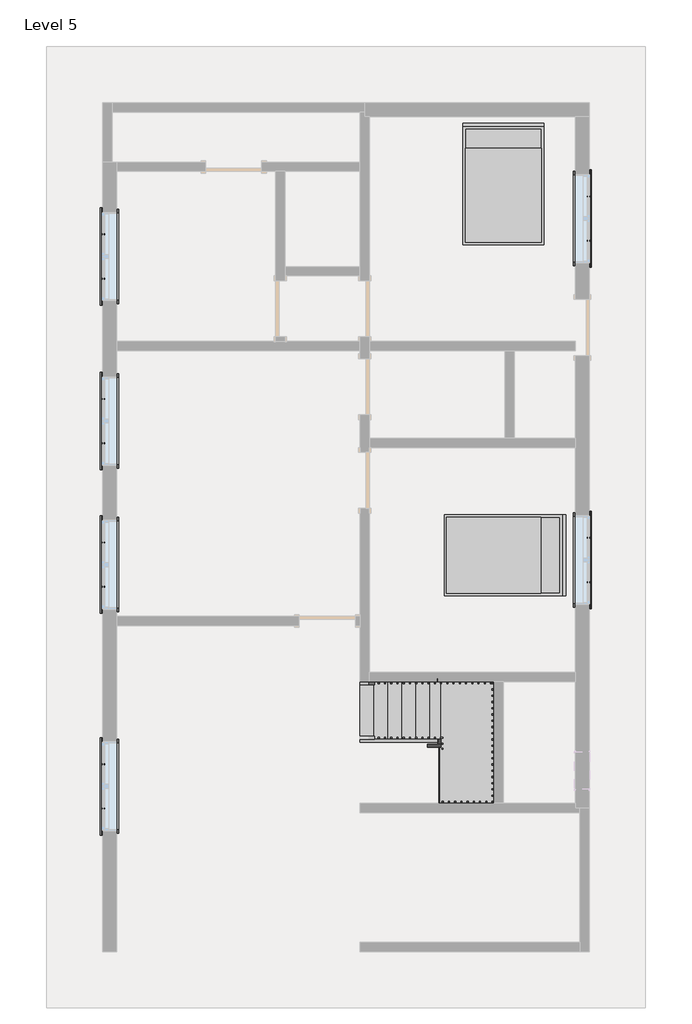
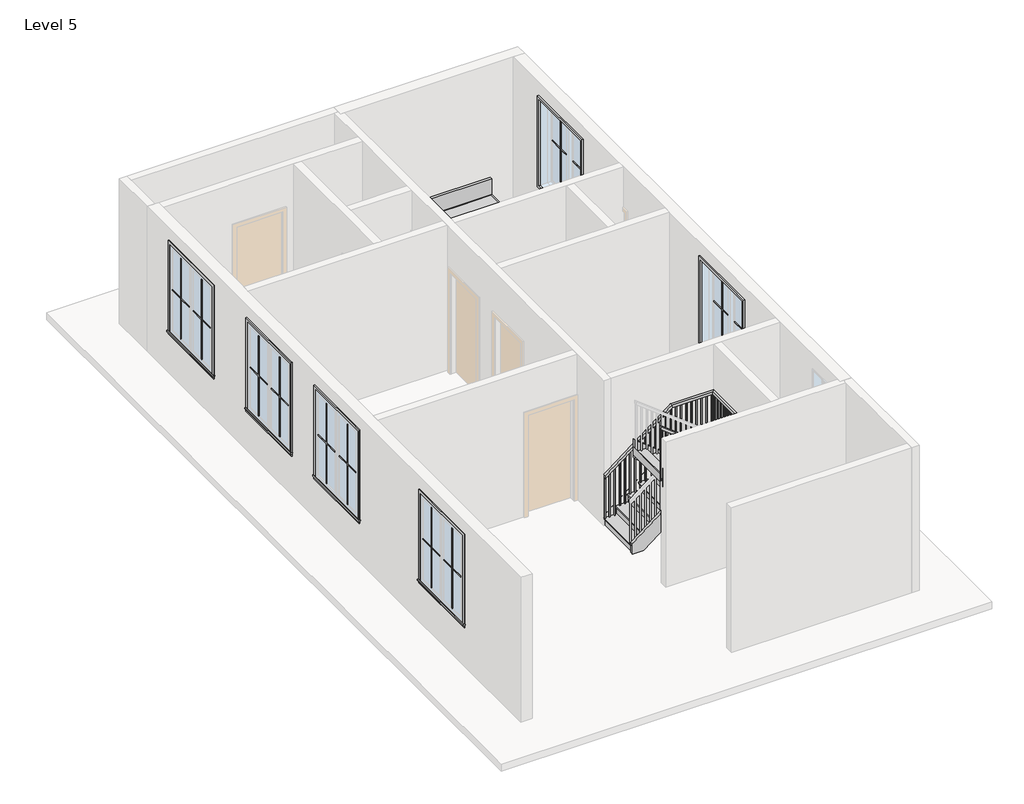
# One storey, part 2 of 2: 24 proxies, 6 members, 2 furniture elements, 1 railing, 1 stair flight.
"""IFC4 building model written with IfcOpenShell, lengths in millimetres."""

from ifc_helpers import new_model, si_unit, frame, origin, place, context, project, spatial, polyline, outline, extrude, faceted_brep, transform, mapped, element, save
from components import muntin_pattern_2x2_muntin_pattern_2x2_bff912c5, muntin_pattern_2x2_muntin_pattern_2x2_c2194282, trim_window_exterior_flat_with_sill_e04b3088, trim_window_interior_flat_picture_frame_2a7685fe, bed_17739_bed_17739_15c61121, stair_flight_8cfd25ce

model = new_model("IFC4")

# Units and contexts
model_context = context("Model", 3, world=origin())
ifc_project = project(units=[si_unit("LENGTHUNIT", "METRE", prefix="MILLI")], contexts=[model_context])

# Site, building, storey
site = spatial("IfcSite", under=ifc_project)
building = spatial("IfcBuilding", under=site)
storey = spatial("IfcBuildingStorey", under=building, Name="Level 5", Elevation=9601.2)

# Proxies
placement = place(None, origin())
muntin_pattern_2x2_muntin_pattern_2x2_shape = muntin_pattern_2x2_muntin_pattern_2x2_bff912c5(model_context)
element("IfcBuildingElementProxy", 1, Name="Muntin Pattern_2x2 : Muntin Pattern_2x2", ObjectType="Muntin Pattern_2x2 : Muntin Pattern_2x2", at=placement, inside=storey, context=model_context, shape_type="MappedRepresentation", body=[
    mapped(muntin_pattern_2x2_muntin_pattern_2x2_shape, transform((-5204.1165352, 3633.8812696, 10585.45), x_axis=(0.0, 1.0, 0.0), y_axis=(-1.0, 0.0, 0.0), z_axis=(0.0, 0.0, 1.0))),
])
element("IfcBuildingElementProxy", 2, Name="Muntin Pattern_2x2 : Muntin Pattern_2x2", ObjectType="Muntin Pattern_2x2 : Muntin Pattern_2x2", at=placement, inside=storey, context=model_context, shape_type="MappedRepresentation", body=[
    mapped(muntin_pattern_2x2_muntin_pattern_2x2_shape, transform((2701.6334648, 4971.3355313, 10585.45), x_axis=(0.0, -1.0, 0.0), y_axis=(1.0, 0.0, 0.0), z_axis=(0.0, 0.0, 1.0))),
])
element("IfcBuildingElementProxy", 3, Name="Muntin Pattern_2x2 : Muntin Pattern_2x2", ObjectType="Muntin Pattern_2x2 : Muntin Pattern_2x2", at=placement, inside=storey, context=model_context, shape_type="MappedRepresentation", body=[
    mapped(muntin_pattern_2x2_muntin_pattern_2x2_shape, transform((2701.6334648, -584.9144687, 10585.45), x_axis=(0.0, -1.0, 0.0), y_axis=(1.0, 0.0, 0.0), z_axis=(0.0, 0.0, 1.0))),
])
element("IfcBuildingElementProxy", 4, Name="Muntin Pattern_2x2 : Muntin Pattern_2x2", ObjectType="Muntin Pattern_2x2 : Muntin Pattern_2x2", at=placement, inside=storey, context=model_context, shape_type="MappedRepresentation", body=[
    mapped(muntin_pattern_2x2_muntin_pattern_2x2_shape, transform((-5204.1165352, 954.9605313, 10585.45), x_axis=(0.0, 1.0, 0.0), y_axis=(-1.0, 0.0, 0.0), z_axis=(0.0, 0.0, 1.0))),
])
element("IfcBuildingElementProxy", 5, Name="Muntin Pattern_2x2 : Muntin Pattern_2x2", ObjectType="Muntin Pattern_2x2 : Muntin Pattern_2x2", at=placement, inside=storey, context=model_context, shape_type="MappedRepresentation", body=[
    mapped(muntin_pattern_2x2_muntin_pattern_2x2_shape, transform((-5204.1165352, -1381.8394687, 10585.45), x_axis=(0.0, 1.0, 0.0), y_axis=(-1.0, 0.0, 0.0), z_axis=(0.0, 0.0, 1.0))),
])
element("IfcBuildingElementProxy", 6, Name="Muntin Pattern_2x2 : Muntin Pattern_2x2", ObjectType="Muntin Pattern_2x2 : Muntin Pattern_2x2", at=placement, inside=storey, context=model_context, shape_type="MappedRepresentation", body=[
    mapped(muntin_pattern_2x2_muntin_pattern_2x2_shape, transform((-5204.1165352, -4988.6394687, 10585.45), x_axis=(0.0, 1.0, 0.0), y_axis=(-1.0, 0.0, 0.0), z_axis=(0.0, 0.0, 1.0))),
])
muntin_pattern_2x2_muntin_pattern_2x2_2_shape = muntin_pattern_2x2_muntin_pattern_2x2_c2194282(model_context)
element("IfcBuildingElementProxy", 7, Name="Muntin Pattern_2x2 : Muntin Pattern_2x2", ObjectType="Muntin Pattern_2x2 : Muntin Pattern_2x2", at=placement, inside=storey, context=model_context, shape_type="MappedRepresentation", body=[
    mapped(muntin_pattern_2x2_muntin_pattern_2x2_2_shape, transform((-5204.1165352, 4354.6062696, 10585.45), x_axis=(0.0, -1.0, 0.0), y_axis=(1.0, 0.0, 0.0), z_axis=(0.0, 0.0, 1.0))),
])
element("IfcBuildingElementProxy", 8, Name="Muntin Pattern_2x2 : Muntin Pattern_2x2", ObjectType="Muntin Pattern_2x2 : Muntin Pattern_2x2", at=placement, inside=storey, context=model_context, shape_type="MappedRepresentation", body=[
    mapped(muntin_pattern_2x2_muntin_pattern_2x2_2_shape, transform((2701.6334648, 4250.6105313, 10585.45), x_axis=(0.0, 1.0, 0.0), y_axis=(-1.0, 0.0, 0.0), z_axis=(0.0, 0.0, 1.0))),
])
element("IfcBuildingElementProxy", 9, Name="Muntin Pattern_2x2 : Muntin Pattern_2x2", ObjectType="Muntin Pattern_2x2 : Muntin Pattern_2x2", at=placement, inside=storey, context=model_context, shape_type="MappedRepresentation", body=[
    mapped(muntin_pattern_2x2_muntin_pattern_2x2_2_shape, transform((2701.6334648, -1305.6394687, 10585.45), x_axis=(0.0, 1.0, 0.0), y_axis=(-1.0, 0.0, 0.0), z_axis=(0.0, 0.0, 1.0))),
])
element("IfcBuildingElementProxy", 10, Name="Muntin Pattern_2x2 : Muntin Pattern_2x2", ObjectType="Muntin Pattern_2x2 : Muntin Pattern_2x2", at=placement, inside=storey, context=model_context, shape_type="MappedRepresentation", body=[
    mapped(muntin_pattern_2x2_muntin_pattern_2x2_2_shape, transform((-5204.1165352, 1675.6855313, 10585.45), x_axis=(0.0, -1.0, 0.0), y_axis=(1.0, 0.0, 0.0), z_axis=(0.0, 0.0, 1.0))),
])
element("IfcBuildingElementProxy", 11, Name="Muntin Pattern_2x2 : Muntin Pattern_2x2", ObjectType="Muntin Pattern_2x2 : Muntin Pattern_2x2", at=placement, inside=storey, context=model_context, shape_type="MappedRepresentation", body=[
    mapped(muntin_pattern_2x2_muntin_pattern_2x2_2_shape, transform((-5204.1165352, -661.1144687, 10585.45), x_axis=(0.0, -1.0, 0.0), y_axis=(1.0, 0.0, 0.0), z_axis=(0.0, 0.0, 1.0))),
])
element("IfcBuildingElementProxy", 12, Name="Muntin Pattern_2x2 : Muntin Pattern_2x2", ObjectType="Muntin Pattern_2x2 : Muntin Pattern_2x2", at=placement, inside=storey, context=model_context, shape_type="MappedRepresentation", body=[
    mapped(muntin_pattern_2x2_muntin_pattern_2x2_2_shape, transform((-5204.1165352, -4267.9144687, 10585.45), x_axis=(0.0, -1.0, 0.0), y_axis=(1.0, 0.0, 0.0), z_axis=(0.0, 0.0, 1.0))),
])
trim_window_exterior_flat_with_sill_shape = trim_window_exterior_flat_with_sill_e04b3088(model_context)
element("IfcBuildingElementProxy", 13, Name="Trim-Window-Exterior-Flat : with Sill", ObjectType="Trim-Window-Exterior-Flat : with Sill", at=placement, inside=storey, context=model_context, shape_type="MappedRepresentation", body=[
    mapped(trim_window_exterior_flat_with_sill_shape, transform((-5213.6415352, 3994.2437696, 12344.4), x_axis=(0.0, -1.0, 0.0), y_axis=(0.0, 0.0, 1.0), z_axis=(-1.0, 0.0, 0.0))),
])
element("IfcBuildingElementProxy", 14, Name="Trim-Window-Exterior-Flat : with Sill", ObjectType="Trim-Window-Exterior-Flat : with Sill", at=placement, inside=storey, context=model_context, shape_type="MappedRepresentation", body=[
    mapped(trim_window_exterior_flat_with_sill_shape, transform((2711.1584648, 4610.9730313, 12344.4), x_axis=(0.0, 1.0, 0.0), y_axis=(0.0, 0.0, 1.0), z_axis=(1.0, 0.0, 0.0))),
])
element("IfcBuildingElementProxy", 15, Name="Trim-Window-Exterior-Flat : with Sill", ObjectType="Trim-Window-Exterior-Flat : with Sill", at=placement, inside=storey, context=model_context, shape_type="MappedRepresentation", body=[
    mapped(trim_window_exterior_flat_with_sill_shape, transform((2711.1584648, -945.2769687, 12344.4), x_axis=(0.0, 1.0, 0.0), y_axis=(0.0, 0.0, 1.0), z_axis=(1.0, 0.0, 0.0))),
])
element("IfcBuildingElementProxy", 16, Name="Trim-Window-Exterior-Flat : with Sill", ObjectType="Trim-Window-Exterior-Flat : with Sill", at=placement, inside=storey, context=model_context, shape_type="MappedRepresentation", body=[
    mapped(trim_window_exterior_flat_with_sill_shape, transform((-5213.6415352, 1315.3230313, 12344.4), x_axis=(0.0, -1.0, 0.0), y_axis=(0.0, 0.0, 1.0), z_axis=(-1.0, 0.0, 0.0))),
])
element("IfcBuildingElementProxy", 17, Name="Trim-Window-Exterior-Flat : with Sill", ObjectType="Trim-Window-Exterior-Flat : with Sill", at=placement, inside=storey, context=model_context, shape_type="MappedRepresentation", body=[
    mapped(trim_window_exterior_flat_with_sill_shape, transform((-5213.6415352, -1021.4769687, 12344.4), x_axis=(0.0, -1.0, 0.0), y_axis=(0.0, 0.0, 1.0), z_axis=(-1.0, 0.0, 0.0))),
])
element("IfcBuildingElementProxy", 18, Name="Trim-Window-Exterior-Flat : with Sill", ObjectType="Trim-Window-Exterior-Flat : with Sill", at=placement, inside=storey, context=model_context, shape_type="MappedRepresentation", body=[
    mapped(trim_window_exterior_flat_with_sill_shape, transform((-5213.6415352, -4628.2769687, 12344.4), x_axis=(0.0, -1.0, 0.0), y_axis=(0.0, 0.0, 1.0), z_axis=(-1.0, 0.0, 0.0))),
])
trim_window_interior_flat_picture_frame_shape = trim_window_interior_flat_picture_frame_2a7685fe(model_context)
element("IfcBuildingElementProxy", 19, Name="Trim-Window-Interior-Flat : Picture Frame", ObjectType="Trim-Window-Interior-Flat : Picture Frame", at=placement, inside=storey, context=model_context, shape_type="MappedRepresentation", body=[
    mapped(trim_window_interior_flat_picture_frame_shape, transform((-4985.0415352, 3994.2437696, 12344.4), x_axis=(0.0, 1.0, 0.0), y_axis=(0.0, 0.0, 1.0), z_axis=(1.0, 0.0, 0.0))),
])
element("IfcBuildingElementProxy", 20, Name="Trim-Window-Interior-Flat : Picture Frame", ObjectType="Trim-Window-Interior-Flat : Picture Frame", at=placement, inside=storey, context=model_context, shape_type="MappedRepresentation", body=[
    mapped(trim_window_interior_flat_picture_frame_shape, transform((2482.5584648, 4610.9730313, 12344.4), x_axis=(0.0, -1.0, 0.0), y_axis=(0.0, 0.0, 1.0), z_axis=(-1.0, 0.0, 0.0))),
])
element("IfcBuildingElementProxy", 21, Name="Trim-Window-Interior-Flat : Picture Frame", ObjectType="Trim-Window-Interior-Flat : Picture Frame", at=placement, inside=storey, context=model_context, shape_type="MappedRepresentation", body=[
    mapped(trim_window_interior_flat_picture_frame_shape, transform((2482.5584648, -945.2769687, 12344.4), x_axis=(0.0, -1.0, 0.0), y_axis=(0.0, 0.0, 1.0), z_axis=(-1.0, 0.0, 0.0))),
])
element("IfcBuildingElementProxy", 22, Name="Trim-Window-Interior-Flat : Picture Frame", ObjectType="Trim-Window-Interior-Flat : Picture Frame", at=placement, inside=storey, context=model_context, shape_type="MappedRepresentation", body=[
    mapped(trim_window_interior_flat_picture_frame_shape, transform((-4985.0415352, 1315.3230313, 12344.4), x_axis=(0.0, 1.0, 0.0), y_axis=(0.0, 0.0, 1.0), z_axis=(1.0, 0.0, 0.0))),
])
element("IfcBuildingElementProxy", 23, Name="Trim-Window-Interior-Flat : Picture Frame", ObjectType="Trim-Window-Interior-Flat : Picture Frame", at=placement, inside=storey, context=model_context, shape_type="MappedRepresentation", body=[
    mapped(trim_window_interior_flat_picture_frame_shape, transform((-4985.0415352, -1021.4769687, 12344.4), x_axis=(0.0, 1.0, 0.0), y_axis=(0.0, 0.0, 1.0), z_axis=(1.0, 0.0, 0.0))),
])
element("IfcBuildingElementProxy", 24, Name="Trim-Window-Interior-Flat : Picture Frame", ObjectType="Trim-Window-Interior-Flat : Picture Frame", at=placement, inside=storey, context=model_context, shape_type="MappedRepresentation", body=[
    mapped(trim_window_interior_flat_picture_frame_shape, transform((-4985.0415352, -4628.2769687, 12344.4), x_axis=(0.0, 1.0, 0.0), y_axis=(0.0, 0.0, 1.0), z_axis=(1.0, 0.0, 0.0))),
])

# Furniture
bed_17739_bed_17739_shape = bed_17739_bed_17739_15c61121(model_context)
element("IfcFurniture", 25, ObjectType="Bed_17739 : Bed_17739", at=placement, inside=storey, context=model_context, shape_type="MappedRepresentation", body=[
    mapped(bed_17739_bed_17739_shape, transform((1314.1584648, 5149.1645078, 9601.2), x_axis=(1.0, 0.0, 0.0), y_axis=(0.0, 1.0, 0.0), z_axis=(0.0, 0.0, 1.0))),
])
element("IfcFurniture", 26, ObjectType="Bed_17739 : Bed_17739", at=placement, inside=storey, context=model_context, shape_type="MappedRepresentation", body=[
    mapped(bed_17739_bed_17739_shape, transform((1314.1584648, -869.0769687, 9601.2), x_axis=(0.0, -1.0, 0.0), y_axis=(1.0, 0.0, 0.0), z_axis=(0.0, 0.0, 1.0))),
])

# Members
element("IfcMember", 27, ObjectType="Stringer - 2\" Width", at=placement, inside=storey, context=model_context, shape_type="SweptSolid", body=[
    extrude(outline(polyline([(9822.9399812, -1022.6415352), (9601.2, -1022.6415352), (9601.2, -811.2687863), (10862.7333333, 810.8400359), (10862.7333333, 314.3488758), (9822.9399812, -1022.6415352)])), frame((0.0, -2926.4769687, 0.0), z_axis=(0.0, 1.0, 0.0), x_axis=(0.0, 0.0, 1.0)), (0.0, 0.0, 1.0), 50.8),
])
element("IfcMember", 28, ObjectType="Stringer - 2\" Width", at=placement, inside=storey, context=model_context, shape_type="SweptSolid", body=[
    extrude(outline(polyline([(1161.7584648, -2875.6769687), (1212.5584648, -2875.6769687), (1212.5584648, -4907.6769687), (1161.7584648, -4907.6769687), (1161.7584648, -2875.6769687)])), frame((0.0, 0.0, 10557.9333333), z_axis=(0.0, 0.0, 1.0), x_axis=(1.0, 0.0, 0.0)), (0.0, 0.0, 1.0), 304.8),
])
element("IfcMember", 29, ObjectType="Stringer - 2\" Width", at=placement, inside=storey, context=model_context, shape_type="SweptSolid", body=[
    extrude(outline(polyline([(10557.9333333, 884.5469698), (12041.1765283, -1022.6415352), (11655.0494451, -1022.6415352), (10557.9333333, 388.0558097), (10557.9333333, 884.5469698)])), frame((0.0, -4958.4769687, 0.0), z_axis=(0.0, 1.0, 0.0), x_axis=(0.0, 0.0, 1.0)), (0.0, 0.0, 1.0), 50.8),
])
element("IfcMember", 30, ObjectType="Stringer - 2\" Width", at=placement, inside=storey, context=model_context, shape_type="SweptSolid", body=[
    extrude(outline(polyline([(9822.9399812, -1022.6415352), (9601.2, -1022.6415352), (9601.2, -811.2687863), (10421.7567404, 243.8221038), (10807.8838236, 243.8221038), (9822.9399812, -1022.6415352)])), frame((0.0, -3912.0539367, 0.0), z_axis=(0.0, 1.0, 0.0), x_axis=(0.0, 0.0, 1.0)), (0.0, 0.0, 1.0), 50.8),
])
element("IfcMember", 31, ObjectType="Stringer - 2\" Width", at=placement, inside=storey, context=model_context, shape_type="SweptSolid", body=[
    extrude(outline(polyline([(243.8221038, -3861.2539367), (294.6221038, -3861.2539367), (294.6221038, -3942.4769687), (243.8221038, -3942.4769687), (243.8221038, -3861.2539367)])), frame((0.0, 0.0, 10557.9333333), z_axis=(0.0, 0.0, 1.0), x_axis=(1.0, 0.0, 0.0)), (0.0, 0.0, 1.0), 304.8),
])
element("IfcMember", 32, ObjectType="Stringer - 2\" Width", at=placement, inside=storey, context=model_context, shape_type="SweptSolid", body=[
    extrude(outline(polyline([(10630.5978382, 294.6221038), (11016.7249214, 294.6221038), (12041.1765283, -1022.6415352), (11655.0494451, -1022.6415352), (10630.5978382, 294.6221038)])), frame((0.0, -3993.2769687, 0.0), z_axis=(0.0, 1.0, 0.0), x_axis=(0.0, 0.0, 1.0)), (0.0, 0.0, 1.0), 50.8),
])

# Railing
element("IfcRailing", 33, ObjectType="Handrail - Rectangular", at=placement, inside=storey, context=model_context, shape_type="SolidModel", body=[
    faceted_brep([(-1022.6415352, -2926.4769687, 10684.9333333), (-1022.6415352, -2926.4769687, 10620.7783974), (-1022.6415352, -2977.2769687, 10620.7783974), (-1022.6415352, -2977.2769687, 10684.9333333), (294.6221038, -2926.4769687, 11700.9333333), (311.9370364, -2926.4769687, 11650.1333333), (311.9370364, -2977.2769687, 11650.1333333), (294.6221038, -2977.2769687, 11700.9333333), (1161.7584648, -2926.4769687, 11700.9333333), (1161.7584648, -2926.4769687, 11650.1333333), (1110.9584648, -2977.2769687, 11650.1333333), (1110.9584648, -2977.2769687, 11700.9333333), (1161.7584648, -4907.6769687, 11700.9333333), (1161.7584648, -4907.6769687, 11650.1333333), (1110.9584648, -4856.8769687, 11650.1333333), (1110.9584648, -4856.8769687, 11700.9333333), (514.1660437, -4907.6769687, 11700.9333333), (496.8511111, -4907.6769687, 11650.1333333), (496.8511111, -4856.8769687, 11650.1333333), (514.1660437, -4856.8769687, 11700.9333333), (-1022.6415352, -4907.6769687, 12886.2666667), (-1022.6415352, -4856.8769687, 12886.2666667), (-1022.6415352, -4856.8769687, 12822.1117307), (-1022.6415352, -4907.6769687, 12822.1117307)], [[[0, 1, 2, 3]], [[1, 0, 4, 5]], [[2, 1, 5, 6]], [[3, 2, 6, 7]], [[0, 3, 7, 4]], [[5, 4, 8, 9]], [[6, 5, 9, 10]], [[7, 6, 10, 11]], [[4, 7, 11, 8]], [[9, 8, 12, 13]], [[10, 9, 13, 14]], [[11, 10, 14, 15]], [[8, 11, 15, 12]], [[13, 12, 16, 17]], [[14, 13, 17, 18]], [[15, 14, 18, 19]], [[12, 15, 19, 16]], [[20, 21, 22, 23]], [[17, 16, 20, 23]], [[18, 17, 23, 22]], [[19, 18, 22, 21]], [[16, 19, 21, 20]]]),
    extrude(outline(polyline([(12809.8674089, -1006.7665352), (11802.5333333, -1006.7665352), (11802.5333333, -987.7165352), (12795.1742226, -987.7165352), (12809.8674089, -1006.7665352)])), frame((0.0, -4891.8019687, 0.0), z_axis=(0.0, 1.0, 0.0), x_axis=(0.0, 0.0, 1.0)), (0.0, 0.0, 1.0), 19.05),
    extrude(outline(polyline([(12731.5037488, -905.1665352), (11802.5333333, -905.1665352), (11802.5333333, -886.1165352), (12716.8105626, -886.1165352), (12731.5037488, -905.1665352)])), frame((0.0, -4891.8019687, 0.0), z_axis=(0.0, 1.0, 0.0), x_axis=(0.0, 0.0, 1.0)), (0.0, 0.0, 1.0), 19.05),
    extrude(outline(polyline([(12653.1400888, -803.5665352), (11802.5333333, -803.5665352), (11802.5333333, -784.5165352), (12638.4469025, -784.5165352), (12653.1400888, -803.5665352)])), frame((0.0, -4891.8019687, 0.0), z_axis=(0.0, 1.0, 0.0), x_axis=(0.0, 0.0, 1.0)), (0.0, 0.0, 1.0), 19.05),
    extrude(outline(polyline([(12574.7764287, -701.9665352), (11633.2, -701.9665352), (11633.2, -682.9165352), (12560.0832425, -682.9165352), (12574.7764287, -701.9665352)])), frame((0.0, -4891.8019687, 0.0), z_axis=(0.0, 1.0, 0.0), x_axis=(0.0, 0.0, 1.0)), (0.0, 0.0, 1.0), 19.05),
    extrude(outline(polyline([(12496.4127687, -600.3665352), (11633.2, -600.3665352), (11633.2, -581.3165352), (12481.7195824, -581.3165352), (12496.4127687, -600.3665352)])), frame((0.0, -4891.8019687, 0.0), z_axis=(0.0, 1.0, 0.0), x_axis=(0.0, 0.0, 1.0)), (0.0, 0.0, 1.0), 19.05),
    extrude(outline(polyline([(12418.0491086, -498.7665352), (11463.8666667, -498.7665352), (11463.8666667, -479.7165352), (12403.3559224, -479.7165352), (12418.0491086, -498.7665352)])), frame((0.0, -4891.8019687, 0.0), z_axis=(0.0, 1.0, 0.0), x_axis=(0.0, 0.0, 1.0)), (0.0, 0.0, 1.0), 19.05),
    extrude(outline(polyline([(12339.6854486, -397.1665352), (11463.8666667, -397.1665352), (11463.8666667, -378.1165352), (12324.9922623, -378.1165352), (12339.6854486, -397.1665352)])), frame((0.0, -4891.8019687, 0.0), z_axis=(0.0, 1.0, 0.0), x_axis=(0.0, 0.0, 1.0)), (0.0, 0.0, 1.0), 19.05),
    extrude(outline(polyline([(12261.3217885, -295.5665352), (11294.5333333, -295.5665352), (11294.5333333, -276.5165352), (12246.6286023, -276.5165352), (12261.3217885, -295.5665352)])), frame((0.0, -4891.8019687, 0.0), z_axis=(0.0, 1.0, 0.0), x_axis=(0.0, 0.0, 1.0)), (0.0, 0.0, 1.0), 19.05),
    extrude(outline(polyline([(12182.9581285, -193.9665352), (11294.5333333, -193.9665352), (11294.5333333, -174.9165352), (12168.2649422, -174.9165352), (12182.9581285, -193.9665352)])), frame((0.0, -4891.8019687, 0.0), z_axis=(0.0, 1.0, 0.0), x_axis=(0.0, 0.0, 1.0)), (0.0, 0.0, 1.0), 19.05),
    extrude(outline(polyline([(12104.5944684, -92.3665352), (11125.2, -92.3665352), (11125.2, -73.3165352), (12089.9012822, -73.3165352), (12104.5944684, -92.3665352)])), frame((0.0, -4891.8019687, 0.0), z_axis=(0.0, 1.0, 0.0), x_axis=(0.0, 0.0, 1.0)), (0.0, 0.0, 1.0), 19.05),
    extrude(outline(polyline([(12026.2308084, 9.2334648), (11125.2, 9.2334648), (11125.2, 28.2834648), (12011.5376221, 28.2834648), (12026.2308084, 9.2334648)])), frame((0.0, -4891.8019687, 0.0), z_axis=(0.0, 1.0, 0.0), x_axis=(0.0, 0.0, 1.0)), (0.0, 0.0, 1.0), 19.05),
    extrude(outline(polyline([(11947.8671484, 110.8334648), (11125.2, 110.8334648), (11125.2, 129.8834648), (11933.1739621, 129.8834648), (11947.8671484, 110.8334648)])), frame((0.0, -4891.8019687, 0.0), z_axis=(0.0, 1.0, 0.0), x_axis=(0.0, 0.0, 1.0)), (0.0, 0.0, 1.0), 19.05),
    extrude(outline(polyline([(11869.5034883, 212.4334648), (10955.8666667, 212.4334648), (10955.8666667, 231.4834648), (11854.8103021, 231.4834648), (11869.5034883, 212.4334648)])), frame((0.0, -4891.8019687, 0.0), z_axis=(0.0, 1.0, 0.0), x_axis=(0.0, 0.0, 1.0)), (0.0, 0.0, 1.0), 19.05),
    extrude(outline(polyline([(11791.1398283, 314.0334648), (10786.5333333, 314.0334648), (10786.5333333, 333.0834648), (11776.446642, 333.0834648), (11791.1398283, 314.0334648)])), frame((0.0, -4891.8019687, 0.0), z_axis=(0.0, 1.0, 0.0), x_axis=(0.0, 0.0, 1.0)), (0.0, 0.0, 1.0), 19.05),
    extrude(outline(polyline([(11712.7761682, 415.6334648), (10786.5333333, 415.6334648), (10786.5333333, 434.6834648), (11698.082982, 434.6834648), (11712.7761682, 415.6334648)])), frame((0.0, -4891.8019687, 0.0), z_axis=(0.0, 1.0, 0.0), x_axis=(0.0, 0.0, 1.0)), (0.0, 0.0, 1.0), 19.05),
    extrude(outline(polyline([(536.2834648, -4891.8019687), (517.2334648, -4891.8019687), (517.2334648, -4872.7519687), (536.2834648, -4872.7519687), (536.2834648, -4891.8019687)])), frame((0.0, 0.0, 10786.5333333), z_axis=(0.0, 0.0, 1.0), x_axis=(1.0, 0.0, 0.0)), (0.0, 0.0, 1.0), 863.6),
    extrude(outline(polyline([(637.8834648, -4891.8019687), (618.8334648, -4891.8019687), (618.8334648, -4872.7519687), (637.8834648, -4872.7519687), (637.8834648, -4891.8019687)])), frame((0.0, 0.0, 10786.5333333), z_axis=(0.0, 0.0, 1.0), x_axis=(1.0, 0.0, 0.0)), (0.0, 0.0, 1.0), 863.6),
    extrude(outline(polyline([(739.4834648, -4891.8019687), (720.4334648, -4891.8019687), (720.4334648, -4872.7519687), (739.4834648, -4872.7519687), (739.4834648, -4891.8019687)])), frame((0.0, 0.0, 10786.5333333), z_axis=(0.0, 0.0, 1.0), x_axis=(1.0, 0.0, 0.0)), (0.0, 0.0, 1.0), 863.6),
    extrude(outline(polyline([(841.0834648, -4891.8019687), (822.0334648, -4891.8019687), (822.0334648, -4872.7519687), (841.0834648, -4872.7519687), (841.0834648, -4891.8019687)])), frame((0.0, 0.0, 10786.5333333), z_axis=(0.0, 0.0, 1.0), x_axis=(1.0, 0.0, 0.0)), (0.0, 0.0, 1.0), 863.6),
    extrude(outline(polyline([(942.6834648, -4891.8019687), (923.6334648, -4891.8019687), (923.6334648, -4872.7519687), (942.6834648, -4872.7519687), (942.6834648, -4891.8019687)])), frame((0.0, 0.0, 10786.5333333), z_axis=(0.0, 0.0, 1.0), x_axis=(1.0, 0.0, 0.0)), (0.0, 0.0, 1.0), 863.6),
    extrude(outline(polyline([(1044.2834648, -4891.8019687), (1025.2334648, -4891.8019687), (1025.2334648, -4872.7519687), (1044.2834648, -4872.7519687), (1044.2834648, -4891.8019687)])), frame((0.0, 0.0, 10786.5333333), z_axis=(0.0, 0.0, 1.0), x_axis=(1.0, 0.0, 0.0)), (0.0, 0.0, 1.0), 863.6),
    extrude(outline(polyline([(1145.8834648, -4771.1519687), (1145.8834648, -4790.2019687), (1126.8334648, -4790.2019687), (1126.8334648, -4771.1519687), (1145.8834648, -4771.1519687)])), frame((0.0, 0.0, 10786.5333333), z_axis=(0.0, 0.0, 1.0), x_axis=(1.0, 0.0, 0.0)), (0.0, 0.0, 1.0), 863.6),
    extrude(outline(polyline([(1145.8834648, -4669.5519687), (1145.8834648, -4688.6019687), (1126.8334648, -4688.6019687), (1126.8334648, -4669.5519687), (1145.8834648, -4669.5519687)])), frame((0.0, 0.0, 10786.5333333), z_axis=(0.0, 0.0, 1.0), x_axis=(1.0, 0.0, 0.0)), (0.0, 0.0, 1.0), 863.6),
    extrude(outline(polyline([(1145.8834648, -4567.9519687), (1145.8834648, -4587.0019687), (1126.8334648, -4587.0019687), (1126.8334648, -4567.9519687), (1145.8834648, -4567.9519687)])), frame((0.0, 0.0, 10786.5333333), z_axis=(0.0, 0.0, 1.0), x_axis=(1.0, 0.0, 0.0)), (0.0, 0.0, 1.0), 863.6),
    extrude(outline(polyline([(1145.8834648, -4466.3519687), (1145.8834648, -4485.4019687), (1126.8334648, -4485.4019687), (1126.8334648, -4466.3519687), (1145.8834648, -4466.3519687)])), frame((0.0, 0.0, 10786.5333333), z_axis=(0.0, 0.0, 1.0), x_axis=(1.0, 0.0, 0.0)), (0.0, 0.0, 1.0), 863.6),
    extrude(outline(polyline([(1145.8834648, -4364.7519687), (1145.8834648, -4383.8019687), (1126.8334648, -4383.8019687), (1126.8334648, -4364.7519687), (1145.8834648, -4364.7519687)])), frame((0.0, 0.0, 10786.5333333), z_axis=(0.0, 0.0, 1.0), x_axis=(1.0, 0.0, 0.0)), (0.0, 0.0, 1.0), 863.6),
    extrude(outline(polyline([(1145.8834648, -4263.1519687), (1145.8834648, -4282.2019687), (1126.8334648, -4282.2019687), (1126.8334648, -4263.1519687), (1145.8834648, -4263.1519687)])), frame((0.0, 0.0, 10786.5333333), z_axis=(0.0, 0.0, 1.0), x_axis=(1.0, 0.0, 0.0)), (0.0, 0.0, 1.0), 863.6),
    extrude(outline(polyline([(1145.8834648, -4161.5519687), (1145.8834648, -4180.6019687), (1126.8334648, -4180.6019687), (1126.8334648, -4161.5519687), (1145.8834648, -4161.5519687)])), frame((0.0, 0.0, 10786.5333333), z_axis=(0.0, 0.0, 1.0), x_axis=(1.0, 0.0, 0.0)), (0.0, 0.0, 1.0), 863.6),
    extrude(outline(polyline([(1145.8834648, -4059.9519687), (1145.8834648, -4079.0019687), (1126.8334648, -4079.0019687), (1126.8334648, -4059.9519687), (1145.8834648, -4059.9519687)])), frame((0.0, 0.0, 10786.5333333), z_axis=(0.0, 0.0, 1.0), x_axis=(1.0, 0.0, 0.0)), (0.0, 0.0, 1.0), 863.6),
    extrude(outline(polyline([(1145.8834648, -3958.3519687), (1145.8834648, -3977.4019687), (1126.8334648, -3977.4019687), (1126.8334648, -3958.3519687), (1145.8834648, -3958.3519687)])), frame((0.0, 0.0, 10786.5333333), z_axis=(0.0, 0.0, 1.0), x_axis=(1.0, 0.0, 0.0)), (0.0, 0.0, 1.0), 863.6),
    extrude(outline(polyline([(1145.8834648, -3856.7519687), (1145.8834648, -3875.8019687), (1126.8334648, -3875.8019687), (1126.8334648, -3856.7519687), (1145.8834648, -3856.7519687)])), frame((0.0, 0.0, 10786.5333333), z_axis=(0.0, 0.0, 1.0), x_axis=(1.0, 0.0, 0.0)), (0.0, 0.0, 1.0), 863.6),
    extrude(outline(polyline([(1145.8834648, -3755.1519687), (1145.8834648, -3774.2019687), (1126.8334648, -3774.2019687), (1126.8334648, -3755.1519687), (1145.8834648, -3755.1519687)])), frame((0.0, 0.0, 10786.5333333), z_axis=(0.0, 0.0, 1.0), x_axis=(1.0, 0.0, 0.0)), (0.0, 0.0, 1.0), 863.6),
    extrude(outline(polyline([(1145.8834648, -3653.5519687), (1145.8834648, -3672.6019687), (1126.8334648, -3672.6019687), (1126.8334648, -3653.5519687), (1145.8834648, -3653.5519687)])), frame((0.0, 0.0, 10786.5333333), z_axis=(0.0, 0.0, 1.0), x_axis=(1.0, 0.0, 0.0)), (0.0, 0.0, 1.0), 863.6),
    extrude(outline(polyline([(1145.8834648, -3551.9519687), (1145.8834648, -3571.0019687), (1126.8334648, -3571.0019687), (1126.8334648, -3551.9519687), (1145.8834648, -3551.9519687)])), frame((0.0, 0.0, 10786.5333333), z_axis=(0.0, 0.0, 1.0), x_axis=(1.0, 0.0, 0.0)), (0.0, 0.0, 1.0), 863.6),
    extrude(outline(polyline([(1145.8834648, -3450.3519687), (1145.8834648, -3469.4019687), (1126.8334648, -3469.4019687), (1126.8334648, -3450.3519687), (1145.8834648, -3450.3519687)])), frame((0.0, 0.0, 10786.5333333), z_axis=(0.0, 0.0, 1.0), x_axis=(1.0, 0.0, 0.0)), (0.0, 0.0, 1.0), 863.6),
    extrude(outline(polyline([(1145.8834648, -3348.7519687), (1145.8834648, -3367.8019687), (1126.8334648, -3367.8019687), (1126.8334648, -3348.7519687), (1145.8834648, -3348.7519687)])), frame((0.0, 0.0, 10786.5333333), z_axis=(0.0, 0.0, 1.0), x_axis=(1.0, 0.0, 0.0)), (0.0, 0.0, 1.0), 863.6),
    extrude(outline(polyline([(1145.8834648, -3247.1519687), (1145.8834648, -3266.2019687), (1126.8334648, -3266.2019687), (1126.8334648, -3247.1519687), (1145.8834648, -3247.1519687)])), frame((0.0, 0.0, 10786.5333333), z_axis=(0.0, 0.0, 1.0), x_axis=(1.0, 0.0, 0.0)), (0.0, 0.0, 1.0), 863.6),
    extrude(outline(polyline([(1145.8834648, -3145.5519687), (1145.8834648, -3164.6019687), (1126.8334648, -3164.6019687), (1126.8334648, -3145.5519687), (1145.8834648, -3145.5519687)])), frame((0.0, 0.0, 10786.5333333), z_axis=(0.0, 0.0, 1.0), x_axis=(1.0, 0.0, 0.0)), (0.0, 0.0, 1.0), 863.6),
    extrude(outline(polyline([(1145.8834648, -3043.9519687), (1145.8834648, -3063.0019687), (1126.8334648, -3063.0019687), (1126.8334648, -3043.9519687), (1145.8834648, -3043.9519687)])), frame((0.0, 0.0, 10786.5333333), z_axis=(0.0, 0.0, 1.0), x_axis=(1.0, 0.0, 0.0)), (0.0, 0.0, 1.0), 863.6),
    extrude(outline(polyline([(1101.4334648, -2942.3519687), (1120.4834648, -2942.3519687), (1120.4834648, -2961.4019687), (1101.4334648, -2961.4019687), (1101.4334648, -2942.3519687)])), frame((0.0, 0.0, 10786.5333333), z_axis=(0.0, 0.0, 1.0), x_axis=(1.0, 0.0, 0.0)), (0.0, 0.0, 1.0), 863.6),
    extrude(outline(polyline([(999.8334648, -2942.3519687), (1018.8834648, -2942.3519687), (1018.8834648, -2961.4019687), (999.8334648, -2961.4019687), (999.8334648, -2942.3519687)])), frame((0.0, 0.0, 10786.5333333), z_axis=(0.0, 0.0, 1.0), x_axis=(1.0, 0.0, 0.0)), (0.0, 0.0, 1.0), 863.6),
    extrude(outline(polyline([(898.2334648, -2942.3519687), (917.2834648, -2942.3519687), (917.2834648, -2961.4019687), (898.2334648, -2961.4019687), (898.2334648, -2942.3519687)])), frame((0.0, 0.0, 10786.5333333), z_axis=(0.0, 0.0, 1.0), x_axis=(1.0, 0.0, 0.0)), (0.0, 0.0, 1.0), 863.6),
    extrude(outline(polyline([(796.6334648, -2942.3519687), (815.6834648, -2942.3519687), (815.6834648, -2961.4019687), (796.6334648, -2961.4019687), (796.6334648, -2942.3519687)])), frame((0.0, 0.0, 10786.5333333), z_axis=(0.0, 0.0, 1.0), x_axis=(1.0, 0.0, 0.0)), (0.0, 0.0, 1.0), 863.6),
    extrude(outline(polyline([(695.0334648, -2942.3519687), (714.0834648, -2942.3519687), (714.0834648, -2961.4019687), (695.0334648, -2961.4019687), (695.0334648, -2942.3519687)])), frame((0.0, 0.0, 10786.5333333), z_axis=(0.0, 0.0, 1.0), x_axis=(1.0, 0.0, 0.0)), (0.0, 0.0, 1.0), 863.6),
    extrude(outline(polyline([(593.4334648, -2942.3519687), (612.4834648, -2942.3519687), (612.4834648, -2961.4019687), (593.4334648, -2961.4019687), (593.4334648, -2942.3519687)])), frame((0.0, 0.0, 10786.5333333), z_axis=(0.0, 0.0, 1.0), x_axis=(1.0, 0.0, 0.0)), (0.0, 0.0, 1.0), 863.6),
    extrude(outline(polyline([(491.8334648, -2942.3519687), (510.8834648, -2942.3519687), (510.8834648, -2961.4019687), (491.8334648, -2961.4019687), (491.8334648, -2942.3519687)])), frame((0.0, 0.0, 10786.5333333), z_axis=(0.0, 0.0, 1.0), x_axis=(1.0, 0.0, 0.0)), (0.0, 0.0, 1.0), 863.6),
    extrude(outline(polyline([(390.2334648, -2942.3519687), (409.2834648, -2942.3519687), (409.2834648, -2961.4019687), (390.2334648, -2961.4019687), (390.2334648, -2942.3519687)])), frame((0.0, 0.0, 10786.5333333), z_axis=(0.0, 0.0, 1.0), x_axis=(1.0, 0.0, 0.0)), (0.0, 0.0, 1.0), 863.6),
    extrude(outline(polyline([(288.6334648, -2942.3519687), (307.6834648, -2942.3519687), (307.6834648, -2961.4019687), (288.6334648, -2961.4019687), (288.6334648, -2942.3519687)])), frame((0.0, 0.0, 10786.5333333), z_axis=(0.0, 0.0, 1.0), x_axis=(1.0, 0.0, 0.0)), (0.0, 0.0, 1.0), 863.6),
    extrude(outline(polyline([(11553.7957248, 187.0334648), (10617.2, 187.0334648), (10617.2, 206.0834648), (11568.4889111, 206.0834648), (11553.7957248, 187.0334648)])), frame((0.0, -2961.4019687, 0.0), z_axis=(0.0, 1.0, 0.0), x_axis=(0.0, 0.0, 1.0)), (0.0, 0.0, 1.0), 19.05),
    extrude(outline(polyline([(11475.4320648, 85.4334648), (10447.8666667, 85.4334648), (10447.8666667, 104.4834648), (11490.125251, 104.4834648), (11475.4320648, 85.4334648)])), frame((0.0, -2961.4019687, 0.0), z_axis=(0.0, 1.0, 0.0), x_axis=(0.0, 0.0, 1.0)), (0.0, 0.0, 1.0), 19.05),
    extrude(outline(polyline([(11397.0684047, -16.1665352), (10447.8666667, -16.1665352), (10447.8666667, 2.8834648), (11411.761591, 2.8834648), (11397.0684047, -16.1665352)])), frame((0.0, -2961.4019687, 0.0), z_axis=(0.0, 1.0, 0.0), x_axis=(0.0, 0.0, 1.0)), (0.0, 0.0, 1.0), 19.05),
    extrude(outline(polyline([(11318.7047447, -117.7665352), (10447.8666667, -117.7665352), (10447.8666667, -98.7165352), (11333.3979309, -98.7165352), (11318.7047447, -117.7665352)])), frame((0.0, -2961.4019687, 0.0), z_axis=(0.0, 1.0, 0.0), x_axis=(0.0, 0.0, 1.0)), (0.0, 0.0, 1.0), 19.05),
    extrude(outline(polyline([(11240.3410846, -219.3665352), (10278.5333333, -219.3665352), (10278.5333333, -200.3165352), (11255.0342709, -200.3165352), (11240.3410846, -219.3665352)])), frame((0.0, -2961.4019687, 0.0), z_axis=(0.0, 1.0, 0.0), x_axis=(0.0, 0.0, 1.0)), (0.0, 0.0, 1.0), 19.05),
    extrude(outline(polyline([(11161.9774246, -320.9665352), (10278.5333333, -320.9665352), (10278.5333333, -301.9165352), (11176.6706109, -301.9165352), (11161.9774246, -320.9665352)])), frame((0.0, -2961.4019687, 0.0), z_axis=(0.0, 1.0, 0.0), x_axis=(0.0, 0.0, 1.0)), (0.0, 0.0, 1.0), 19.05),
    extrude(outline(polyline([(11083.6137645, -422.5665352), (10109.2, -422.5665352), (10109.2, -403.5165352), (11098.3069508, -403.5165352), (11083.6137645, -422.5665352)])), frame((0.0, -2961.4019687, 0.0), z_axis=(0.0, 1.0, 0.0), x_axis=(0.0, 0.0, 1.0)), (0.0, 0.0, 1.0), 19.05),
    extrude(outline(polyline([(11005.2501045, -524.1665352), (10109.2, -524.1665352), (10109.2, -505.1165352), (11019.9432908, -505.1165352), (11005.2501045, -524.1665352)])), frame((0.0, -2961.4019687, 0.0), z_axis=(0.0, 1.0, 0.0), x_axis=(0.0, 0.0, 1.0)), (0.0, 0.0, 1.0), 19.05),
    extrude(outline(polyline([(10926.8864445, -625.7665352), (9939.8666667, -625.7665352), (9939.8666667, -606.7165352), (10941.5796307, -606.7165352), (10926.8864445, -625.7665352)])), frame((0.0, -2961.4019687, 0.0), z_axis=(0.0, 1.0, 0.0), x_axis=(0.0, 0.0, 1.0)), (0.0, 0.0, 1.0), 19.05),
    extrude(outline(polyline([(10848.5227844, -727.3665352), (9939.8666667, -727.3665352), (9939.8666667, -708.3165352), (10863.2159707, -708.3165352), (10848.5227844, -727.3665352)])), frame((0.0, -2961.4019687, 0.0), z_axis=(0.0, 1.0, 0.0), x_axis=(0.0, 0.0, 1.0)), (0.0, 0.0, 1.0), 19.05),
    extrude(outline(polyline([(10770.1591244, -828.9665352), (9770.5333333, -828.9665352), (9770.5333333, -809.9165352), (10784.8523106, -809.9165352), (10770.1591244, -828.9665352)])), frame((0.0, -2961.4019687, 0.0), z_axis=(0.0, 1.0, 0.0), x_axis=(0.0, 0.0, 1.0)), (0.0, 0.0, 1.0), 19.05),
    extrude(outline(polyline([(10691.7954643, -930.5665352), (9770.5333333, -930.5665352), (9770.5333333, -911.5165352), (10706.4886506, -911.5165352), (10691.7954643, -930.5665352)])), frame((0.0, -2961.4019687, 0.0), z_axis=(0.0, 1.0, 0.0), x_axis=(0.0, 0.0, 1.0)), (0.0, 0.0, 1.0), 19.05),
    extrude(outline(polyline([(1145.8834648, -4872.7519687), (1145.8834648, -4891.8019687), (1126.8334648, -4891.8019687), (1126.8334648, -4872.7519687), (1145.8834648, -4872.7519687)])), frame((0.0, 0.0, 10786.5333333), z_axis=(0.0, 0.0, 1.0), x_axis=(1.0, 0.0, 0.0)), (0.0, 0.0, 1.0), 863.6),
    extrude(outline(polyline([(1126.8334648, -2942.3519687), (1145.8834648, -2942.3519687), (1145.8834648, -2961.4019687), (1126.8334648, -2961.4019687), (1126.8334648, -2942.3519687)])), frame((0.0, 0.0, 10786.5333333), z_axis=(0.0, 0.0, 1.0), x_axis=(1.0, 0.0, 0.0)), (0.0, 0.0, 1.0), 863.6),
    extrude(outline(polyline([(12822.1117307, -1022.6415352), (11802.5333333, -1022.6415352), (11802.5333333, -1003.5915352), (12807.4185445, -1003.5915352), (12822.1117307, -1022.6415352)])), frame((0.0, -4891.8019687, 0.0), z_axis=(0.0, 1.0, 0.0), x_axis=(0.0, 0.0, 1.0)), (0.0, 0.0, 1.0), 19.05),
    extrude(outline(polyline([(10620.7783974, -1022.6415352), (9770.5333333, -1022.6415352), (9770.5333333, -1003.5915352), (10635.4715837, -1003.5915352), (10620.7783974, -1022.6415352)])), frame((0.0, -2961.4019687, 0.0), z_axis=(0.0, 1.0, 0.0), x_axis=(0.0, 0.0, 1.0)), (0.0, 0.0, 1.0), 19.05),
])

# Stair flight
stair_flight_shape = stair_flight_8cfd25ce(model_context)
element("IfcStairFlight", 34, ObjectType="2\" Tread 1\" Nosing 1/4\" Riser", at=placement, inside=storey, context=model_context, shape_type="MappedRepresentation", body=[
    mapped(stair_flight_shape, transform((0.0, 0.0, 0.0), x_axis=(1.0, 0.0, 0.0), y_axis=(0.0, 1.0, 0.0), z_axis=(0.0, 0.0, 1.0))),
])

save(model, "model.ifc")

# Revit data of these elements
# Type "Muntin Pattern_2x2 : Muntin Pattern_2x2"
#   Width [instance default] = 4' - 0"
#   Thickness = 0' - 0 1/2"
#   Height [instance default] = 4' - 0"
#   Distance = 0' - 0 3/4"
#   Interior Material [instance default] = none
#   Exterior Material [instance default] = none
#   Default Elevation = 0
# Type "Trim-Window-Exterior-Flat : with Sill"
#   Trim Width = 0' - 2 1/4"
#   Trim Thickness_Picture Frame = 0' - 1 1/4"
#   Trim Thickness_with Sill = 0' - 0 3/4"
#   Sill Thickness = 0' - 1 1/4"
#   Opening Width [instance default] = 2' - 0"
#   Opening Height [instance default] = 3' - 0"
#   Default Elevation = 4' - 0"
#   Sill = yes
#   Picture Frame = no
#   Trim Material [instance default] = none
# Type "Trim-Window-Interior-Flat : Picture Frame"
#   Trim Thickness_Picture Frame = 0' - 1 1/4"
#   Trim Width = 0' - 2 1/4"
#   Trim Thickness_with Sill = 0' - 0 3/4"
#   Sill Thickness = 0' - 1 1/4"
#   Opening Width [instance default] = 2' - 0"
#   Opening Height [instance default] = 3' - 0"
#   Default Elevation = 4' - 0"
#   Sill = no
#   Picture Frame = yes
#   Trim Material [instance default] = none
# Type "Bed_17739 : Bed_17739"
#   Default Elevation = 0
# Type "Handrail - Rectangular"
#   Assembly Code = "C2010400"
#   built-in parameter 1008612 = 0.0416667 (stored number, unit not read)
#   built-in parameter 1008611 = 0.0416667 (stored number, unit not read)
#   built-in parameter 1008609 = 0.333333 (stored number, unit not read)
#   built-in parameter 1008604 = 0.166667 (stored number, unit not read)
#   built-in parameter 1008603 = 0.166667 (stored number, unit not read)
#   Railing Height = 3' - 0"
#   built-in parameter 1008630 = 2
#   built-in parameter 1008610 = 2
#   built-in parameter 1008618 = Baluster - Square : 3/4"
# Elements 1, 2, 3, 4, 5, 6, 7, 8, 9, 10, 11, 12 (IfcBuildingElementProxy, "Muntin Pattern_2x2 : Muntin Pattern_2x2")
#   Width = 1' - 11 1/8"
#   Height = 5' - 6 1/2"
#   Interior Material = Wood - Stained
#   Exterior Material = Clad - White
#   Phase Created = New Construction
#   Materials on its faces: "Clad - White", "Wood - Stained"
# Elements 13, 14, 15, 16, 17, 18 (IfcBuildingElementProxy, "Trim-Window-Exterior-Flat : with Sill")
#   Opening Width = 4' - 9"
#   Opening Height = 6' - 0"
#   Trim Material = Clad - White
#   Phase Created = New Construction
#   Materials on its faces: "Clad - White"
# Elements 19, 20, 21, 22, 23, 24 (IfcBuildingElementProxy, "Trim-Window-Interior-Flat : Picture Frame")
#   Opening Width = 4' - 9"
#   Opening Height = 6' - 0"
#   Trim Material = Wood - Stained
#   Phase Created = New Construction
#   Materials on its faces: "Wood - Stained"
# Elements 25, 26 (IfcFurniture, "Bed_17739 : Bed_17739")
#   Phase Created = New Construction
#   Materials on its faces: "legs", "sheets", "bed frame", "Blanket"
# Elements 27, 28, 29, 30, 31, 32 (IfcMember, "Stringer - 2\" Width")
#   Phase Created = New Construction
# Element 33 (IfcRailing, "Handrail - Rectangular")
#   Phase Created = New Construction
# Element 34 (IfcStairFlight, "2\" Tread 1\" Nosing 1/4\" Riser")
#   Phase Created = New Construction
# Materials
#   "Clad - White": class "Wood", colour RGB 242 242 238, transparency 0, Cost = 0
#   "Wood - Stained": class "Wood", colour RGB 224 178 126, transparency 0, Cost = 0
#   "legs": colour RGB 90 73 37, transparency 0, Cost = 0
#   "sheets": colour RGB 200 195 176, transparency 0, Cost = 0
#   "bed frame": colour RGB 90 73 37, transparency 0, Cost = 0
#   "Blanket": class "System", colour RGB 59 0 1, transparency 0, Cost = 0
